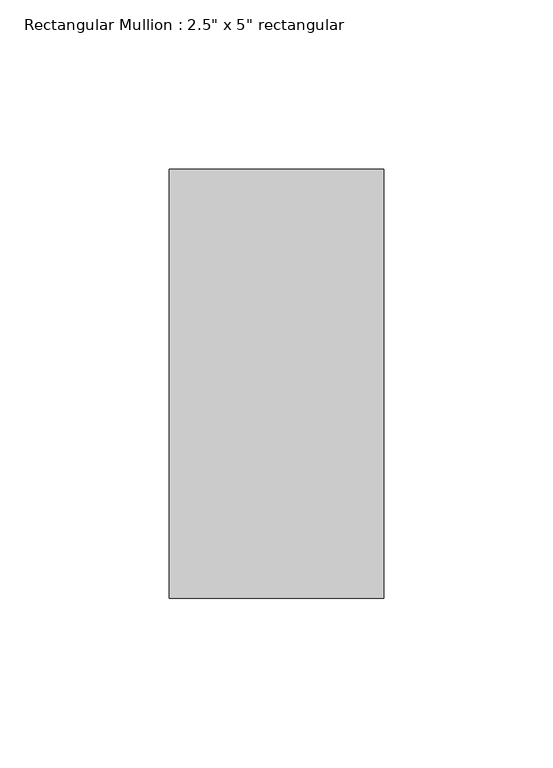
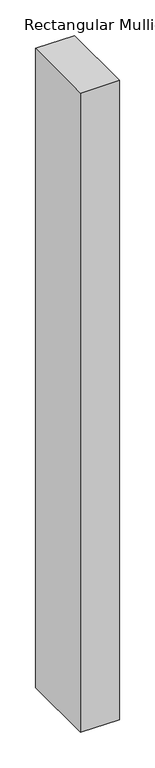
"""IFC4 building model written with IfcOpenShell, lengths in millimetres: member geometry."""

from ifc_helpers import new_model, si_unit, frame, origin, place, context, project, spatial, polyline, outline, extrude, source, transform, mapped, element, save


def member_65519335(model_context):
    return source(origin(), model_context, "Body", "SweptSolid", [
        extrude(outline(polyline([(31.75, 63.5), (31.75, -63.5), (-31.75, -63.5), (-31.75, 63.5), (31.75, 63.5)])), frame((0.0, 0.0, -1098.5500001), z_axis=(0.0, 0.0, 1.0), x_axis=(1.0, 0.0, 0.0)), (0.0, 0.0, 1.0), 1098.5500001),
    ])


if __name__ == "__main__":
    model = new_model("IFC4")
    model_context = context("Model", 3, world=origin())
    ifc_project = project(units=[si_unit("LENGTHUNIT", "METRE", prefix="MILLI")], contexts=[model_context])
    site = spatial("IfcSite", under=ifc_project)
    building = spatial("IfcBuilding", under=site)
    placement = place(None, origin())
    member_shape = member_65519335(model_context)
    element("IfcMember", 1, ObjectType="Rectangular Mullion : 2.5\" x 5\" rectangular", at=placement, inside=building, context=model_context, shape_type="MappedRepresentation", body=[
        mapped(member_shape, transform((0.0, 0.0, 0.0), x_axis=(1.0, 0.0, 0.0), y_axis=(0.0, 1.0, 0.0), z_axis=(0.0, 0.0, 1.0))),
    ])
    save(model, "model.ifc")

# Revit data of these elements
# Type "Rectangular Mullion : 2.5\" x 5\" rectangular"
#   built-in parameter 1007304 = 0.416667 (stored number, unit not read)
#   built-in parameter 1007301 = 0.104167 (stored number, unit not read)
#   built-in parameter 1007300 = 0.104167 (stored number, unit not read)
# Element 1 (IfcMember, "Rectangular Mullion : 2.5\" x 5\" rectangular")
#   Materials on its faces: "BLACK COLOUR"
# Materials
#   "BLACK COLOUR": class "Generic", colour RGB 120 120 120, transparency 0, Cost = 0
